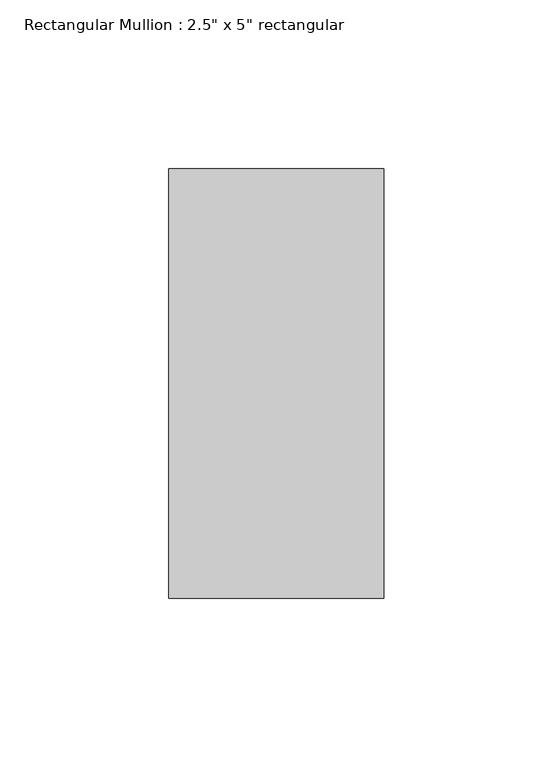
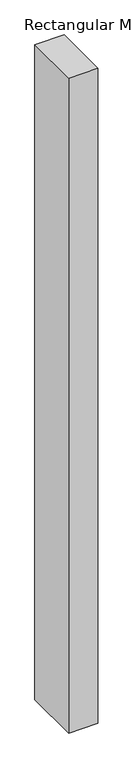
"""IFC4 building model written with IfcOpenShell, lengths in millimetres: member geometry."""

from ifc_helpers import new_model, si_unit, frame, origin, place, context, project, spatial, polyline, outline, extrude, source, transform, mapped, element, save


def member_83f53977(model_context):
    return source(origin(), model_context, "Body", "SweptSolid", [
        extrude(outline(polyline([(0.0, 63.5), (0.0, -63.5), (-63.5, -63.5), (-63.5, 63.5), (0.0, 63.5)])), frame((0.0, 0.0, -1503.5884629), z_axis=(0.0, 0.0, 1.0), x_axis=(1.0, 0.0, 0.0)), (0.0, 0.0, 1.0), 1503.5884629),
    ])


if __name__ == "__main__":
    model = new_model("IFC4")
    model_context = context("Model", 3, world=origin())
    ifc_project = project(units=[si_unit("LENGTHUNIT", "METRE", prefix="MILLI")], contexts=[model_context])
    site = spatial("IfcSite", under=ifc_project)
    building = spatial("IfcBuilding", under=site)
    placement = place(None, origin())
    member_shape = member_83f53977(model_context)
    element("IfcMember", 1, ObjectType="Rectangular Mullion : 2.5\" x 5\" rectangular", at=placement, inside=building, context=model_context, shape_type="MappedRepresentation", body=[
        mapped(member_shape, transform((0.0, 0.0, 0.0), x_axis=(1.0, 0.0, 0.0), y_axis=(0.0, 1.0, 0.0), z_axis=(0.0, 0.0, 1.0))),
    ])
    save(model, "model.ifc")

# Revit data of these elements
# Type "Rectangular Mullion : 2.5\" x 5\" rectangular"
#   built-in parameter 1007304 = 0.416667 (stored number, unit not read)
#   built-in parameter 1007301 = 0.104167 (stored number, unit not read)
#   built-in parameter 1007300 = 0.104167 (stored number, unit not read)
# Element 1 (IfcMember, "Rectangular Mullion : 2.5\" x 5\" rectangular")
#   Materials on its faces: "Aluminum"
# Materials
#   "Aluminum": class "Metal", colour RGB 247 247 247, transparency 0, Description = "Aluminum 6061", Cost = 0
